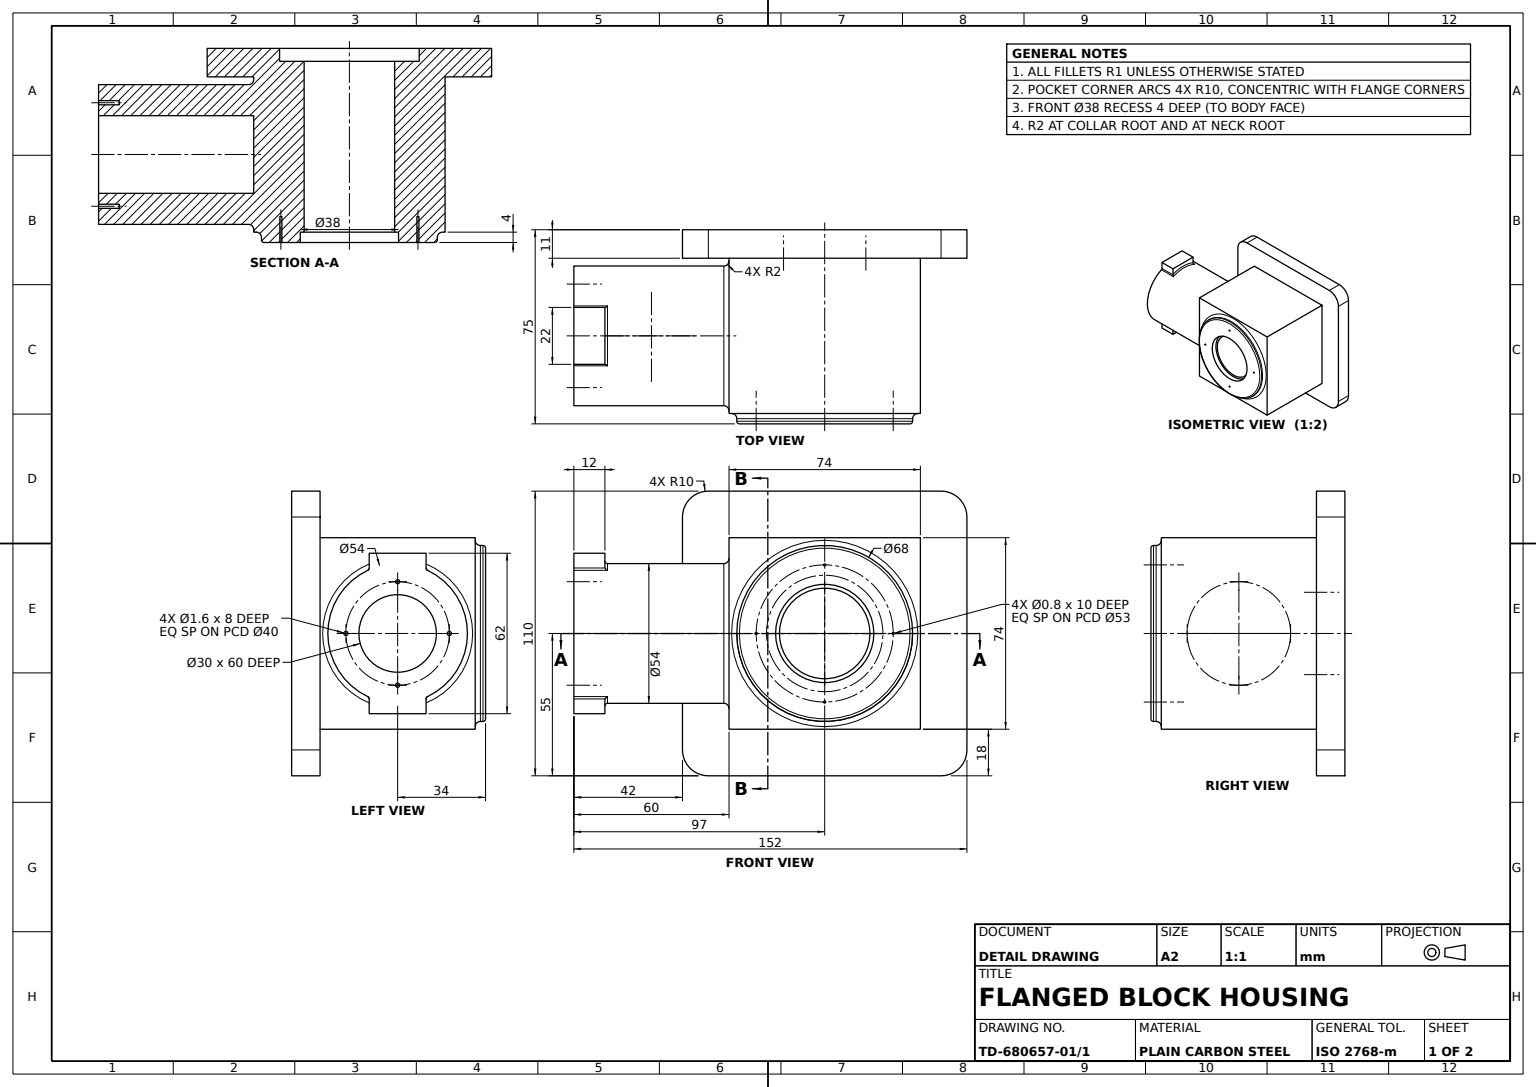
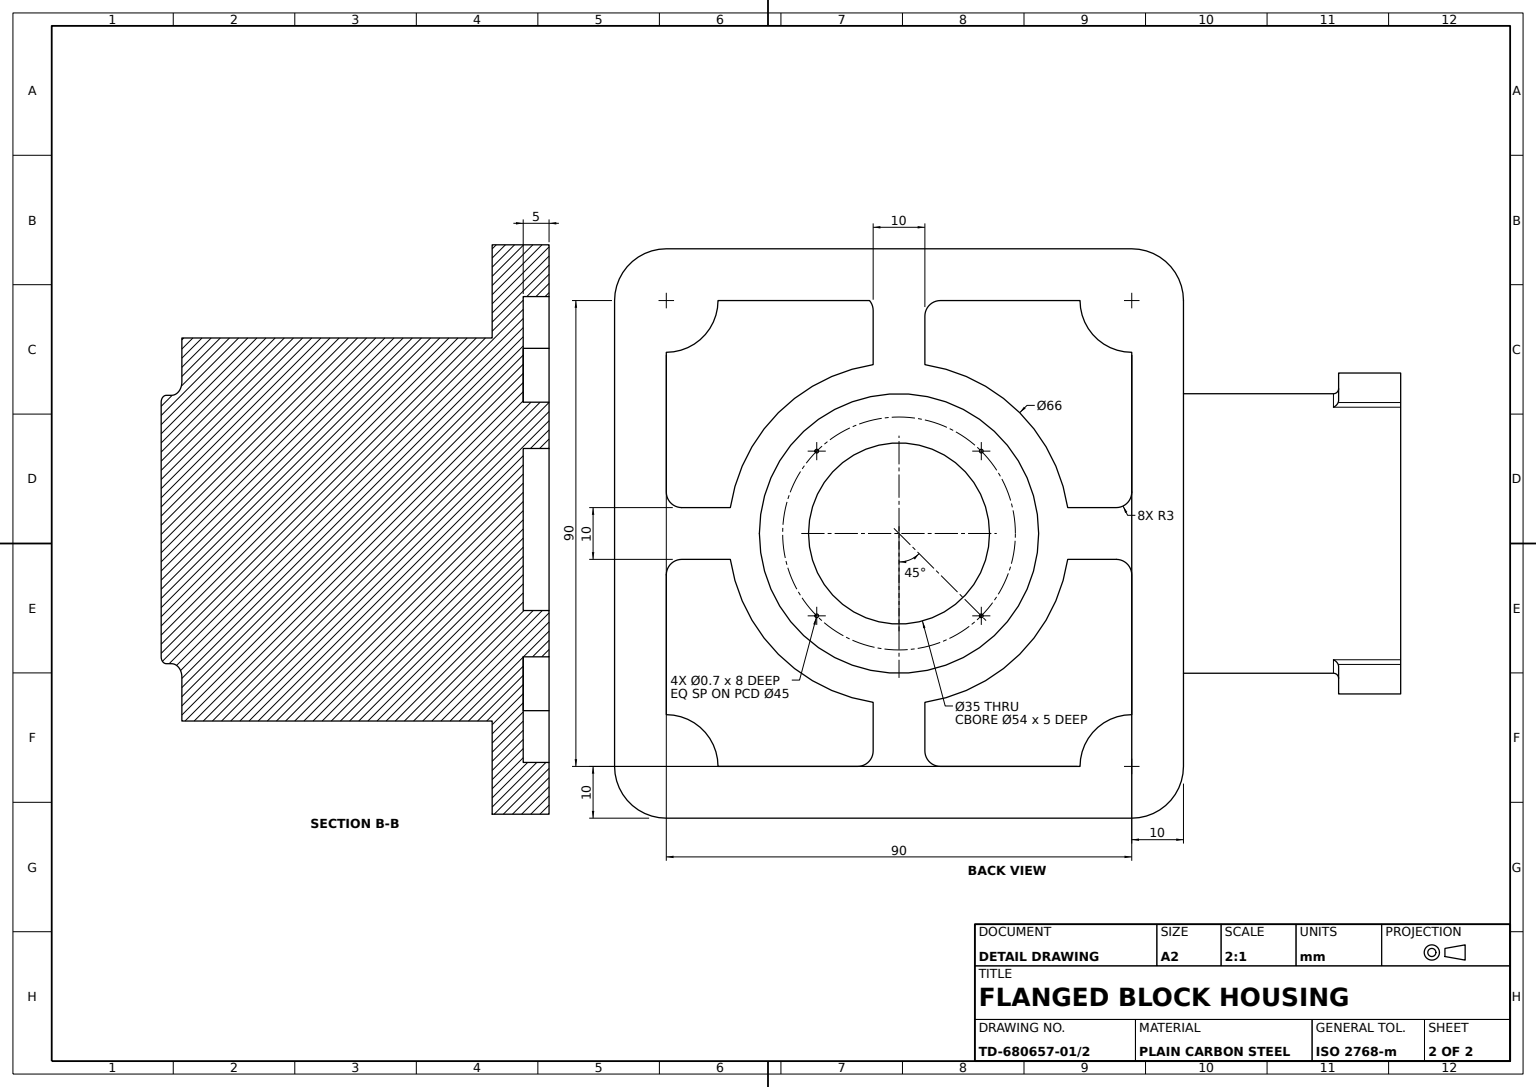
SolidWorks part; units mm, degrees
material "Plain Carbon Steel"
ref_plane "Front Plane" through (0, 0, 0) normal (0, 0, 1) x (1, 0, 0)
ref_plane "Top Plane" through (0, 0, 0) normal (0, 1, 0) x (1, 0, 0)
ref_plane "Right Plane" through (0, 0, 0) normal (1, 0, 0) x (0, 0, -1)
sketch "Mounting Flange Sketch" plane through (0, 0, 0) normal (0, 0, 1) x (1, 0, 0)
  line L0 (0, 0) -> (110, 0)
  line L1 (110, 0) -> (110, 110)
  line L2 (110, 110) -> (0, 110)
  line L3 (0, 110) -> (0, 0)
  dimension "D1" = 110
  dimension "D2" = 110
extrude "Mounting Flange 110x110" add sketch "Mounting Flange Sketch" along normal blind 11
sketch "Flange Recess Sketch" plane through (0, 0, 0) normal (0, 0, -1) x (-1, 0, 0)
  line L0 (-50, 13) -> (-50, 22.381)
  line L14 (-60, 13) -> (-60, 22.381)
  line L15 (-97, 60) -> (-87.619, 60)
  line L16 (-60, 98.0762) -> (-60, 87.619)
  line L17 (-97, 50) -> (-87.619, 50)
  line L18 (-50, 97) -> (-50, 87.619)
  line L19 (-13, 60) -> (-22.381, 60)
  line L21 (-13, 50) -> (-22.381, 50)
  line L24 (-47, 100) -> (-20, 100)
  line L26 (-10, 20) -> (-10, 47)
  line L27 (-10, 63) -> (-10, 90)
  line L30 (-20, 10) -> (-47, 10)
  line L32 (-63, 10) -> (-90, 10)
  line L33 (-100, 47) -> (-100, 20)
  line L35 (-100, 63) -> (-100, 90)
  line L36 (-90, 100) -> (-60.698, 100)
  arc A4 (-50, 22.381) -> (-22.381, 50) centre (-55, 55) ccw
  circle A5 centre (-55, 55) radius 17.5
  circle A6 centre (-55, 55) radius 22.5 construction
  circle A7 centre (-55, 55) radius 27
  arc A8 (-60.698, 100) -> (-60, 98.0762) centre (-63, 98.0762) cw
  arc A9 (-47, 100) -> (-50, 97) centre (-47, 97) ccw
  arc A10 (-13, 60) -> (-10, 63) centre (-13, 63) ccw
  arc A11 (-10, 47) -> (-13, 50) centre (-13, 47) ccw
  arc A12 (-50, 13) -> (-47, 10) centre (-47, 13) ccw
  arc A13 (-63, 10) -> (-60, 13) centre (-63, 13) ccw
  arc A14 (-97, 50) -> (-100, 47) centre (-97, 47) ccw
  arc A15 (-97, 60) -> (-100, 63) centre (-97, 63) cw
  arc A17 (-100, 90) -> (-90, 100) centre (-100, 100) ccw
  arc A18 (-20, 100) -> (-10, 90) centre (-10, 100) ccw
  arc A19 (-10, 20) -> (-20, 10) centre (-10, 10) ccw
  arc A20 (-90, 10) -> (-100, 20) centre (-100, 10) ccw
  arc A21 (-87.619, 50) -> (-60, 22.381) centre (-55, 55) ccw
  arc A22 (-60, 87.619) -> (-87.619, 60) centre (-55, 55) ccw
  arc A23 (-22.381, 60) -> (-50, 87.619) centre (-55, 55) ccw
  point P2 (-100, 10)
  point P11 (-10, 100)
  point P14 (-100, 100)
  dimension "D3" = 3
  dimension "D4" = 66
  dimension "D5" = 35
  dimension "D6" = 45
  dimension "D7" = 54
  dimension "D15" = 3
  dimension "D16" = 3
  dimension "D18" = 3
  dimension "D10" = 3
  dimension "D19" = 3
  dimension "D2" = 3
  dimension "D8" = 3
  dimension "D9" = 20
  dimension "D20" = 20
  dimension "D21" = 10
  dimension "D22" = 10
  dimension "D11" = 100
  dimension "D13" = 90
  dimension "D17" = 45
  dimension "D23" = 45
  dimension "D12" = 10
  dimension "D14" = 90
  dimension "D24" = 10
  dimension "D25" = 5
  dimension "D26" = 10
  dimension "D27" = 5
  dimension "D28" = 10.4572
extrude "Flange Recess" cut sketch "Flange Recess Sketch" against normal blind 5
sketch "Body Block Sketch" plane through (0, 0, 11) normal (0, 0, 1) x (1, 0, 0)
  line L0 (0, 110) -> (0, 0) construction
  line L1 (0, 0) -> (110, 0) construction
  line L2 (55, 18) -> (92, 18)
  line L3 (92, 18) -> (92, 92)
  line L4 (92, 92) -> (18, 92)
  line L5 (18, 92) -> (18, 18)
  line L6 (18, 18) -> (55, 18)
  dimension "D1" = 74
  dimension "D2" = 74
  dimension "D3" = 18
  dimension "D4" = 18
extrude "Body Block 74x74" add sketch "Body Block Sketch" along normal blind 60
sketch "Neck Sketch" plane through (18, 0, 0) normal (-1, 0, 0) x (0, 0, 1)
  line L0 (11, 92) -> (11, 18) construction
  line L1 (71, 18) -> (11, 18) construction
  circle A0 centre (41, 55) radius 27
  dimension "D1" = 54
  dimension "D2" = 30
  dimension "D3" = 37
extrude "Cylindrical Neck Ø54" add sketch "Neck Sketch" along normal blind 60
ref_plane "Plane2" through (0, 28, 0) normal (0, 1, 0) x (1, 0, 0)
ref_plane "Plane4" through (-42, 0, 0) normal (1, 0, 0) x (0, 0, -1)
sketch "Key Lug Sketch" plane through (-42, 0, 0) normal (1, 0, 0) x (0, 0, -1)
  line L1 (-41, 86) -> (-30, 86)
  line L2 (-41, 86) -> (-52, 86)
  line L3 (-52, 86) -> (-52, 79.6577)
  line L4 (-30, 86) -> (-30, 79.6577)
  circle A0 centre (-41, 55) radius 27 construction
  circle A1 centre (-41, 55) radius 27 construction
  arc A2 (-30, 79.6577) -> (-52, 79.6577) centre (-41, 55) ccw
  dimension "D1" = 11
  dimension "D2" = 6.3423
extrude "Neck Key Lug" add sketch "Key Lug Sketch" along normal blind 12
ref_plane "Plane5" through (0, 55, 0) normal (0, 1, 0) x (1, 0, 0)
mirror "Key Lug Mirror" about plane through (0, 55, 0) normal (0, 1, 0) of "Neck Key Lug"
sketch "Neck Bore Sketch" plane through (-42, 0, 0) normal (-1, 0, 0) x (0, 0, 1)
  circle A0 centre (41, 55) radius 15.0005
  dimension "D1" = 30.0009
extrude "Neck Bore Ø30" cut sketch "Neck Bore Sketch" against normal blind 60
sketch "Neck Mark Sketch" plane through (-42, 0, 0) normal (-1, 0, 0) x (0, 0, 1)
  line L0 (41, 55) -> (61, 55) construction
  circle A0 centre (41, 55) radius 20 construction
  circle A1 centre (61, 55) radius 0.8
  dimension "D1" = 40
  dimension "D2" = 1.6
extrude "Neck Mark" cut sketch "Neck Mark Sketch" against normal blind 8
pattern_circular "Neck Mark Pattern 4x" count 4 over 360 about axis through (0, 55, 41) along (1, 0, 0) of "Neck Mark"
sketch "Front Collar Sketch" plane through (0, 0, 71) normal (0, 0, 1) x (1, 0, 0)
  line L0 (18, 92) -> (18, 18) construction
  line L1 (92, 92) -> (18, 92) construction
  circle A0 centre (55, 55) radius 34
  circle A1 centre (55, 55) radius 19
  dimension "D1" = 68
  dimension "D2" = 38
  dimension "D3" = 37
  dimension "D4" = 37
extrude "Front Collar Ring Ø68" add sketch "Front Collar Sketch" along normal blind 4
sketch "Front Bore Sketch" plane through (0, 0, 71) normal (0, 0, 1) x (1, 0, 0)
  circle A0 centre (55, 55) radius 17.5
  dimension "D1" = 35
extrude "Front Bore Ø35" cut sketch "Front Bore Sketch" against normal through all
sketch "Collar Mark Sketch" plane through (0, 0, 75) normal (0, 0, 1) x (1, 0, 0)
  line L0 (55, 55) -> (55, 81.5) construction
  circle A0 centre (55, 55) radius 26.5 construction
  circle A1 centre (55, 81.5) radius 0.4
  dimension "D1" = 53
  dimension "D2" = 0.8
extrude "Collar Mark" cut sketch "Collar Mark Sketch" against normal blind 10
pattern_circular "Collar Mark Pattern 4x" count 4 over 360 about axis through (55, 55, 0) along (0, 0, 1) of "Collar Mark"
sketch "Recess Mark Sketch" plane through (0, 0, 5) normal (0, 0, -1) x (-1, 0, 0)
  line L0 (-55, 55) -> (-55, 77.5) construction
  line L1 (-55, 55) -> (-70.9099, 70.9099) construction
  circle A0 centre (-55, 55) radius 22.5 construction
  circle A1 centre (-70.9099, 70.9099) radius 0.35
  dimension "D1" = 45
  dimension "D3" = 0.7
  dimension "D2" = 45
extrude "Recess Mark" cut sketch "Recess Mark Sketch" against normal blind 8
pattern_circular "Recess Mark Pattern 4x" count 4 over 360 about axis through (55, 55, 0) along (0, 0, 1) of "Recess Mark"
fillet "Flange Corner Fillets R10" radius 10 4 edges at (110, 110, 5.5) (0, 110, 5.5) (0, 0, 5.5) (110, 0, 5.5)
fillet "Collar Edge Fillet R1" radius 1 1 edges at (89, 55, 75)
fillet "Collar Root Fillet R2" radius 2 1 edges at (89, 55, 71)
fillet "Neck Root Fillet R2" radius 2 1 edges at (18, 55, 14)
fillet "Key Lug Fillets R1" radius 1 6 edges at (-36, 30.3423, 30) (-30, 28, 41) (-36, 30.3423, 52) (-36, 79.6577, 30) (-30, 82, 41) (-36, 79.6577, 52)
